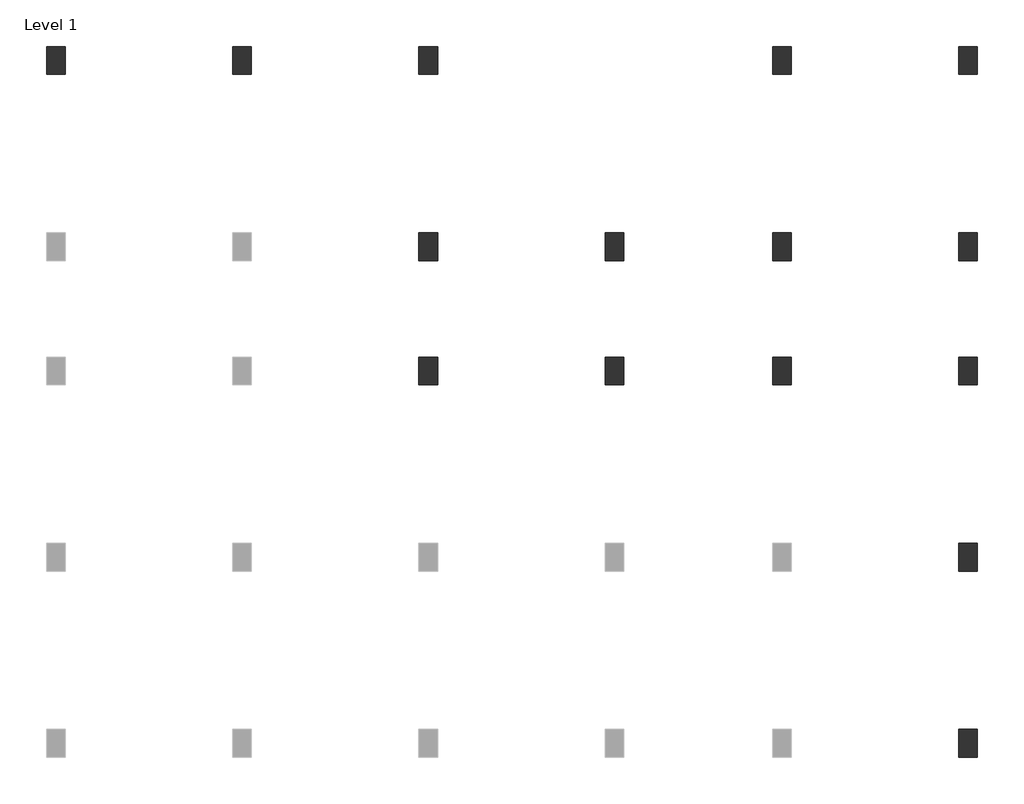
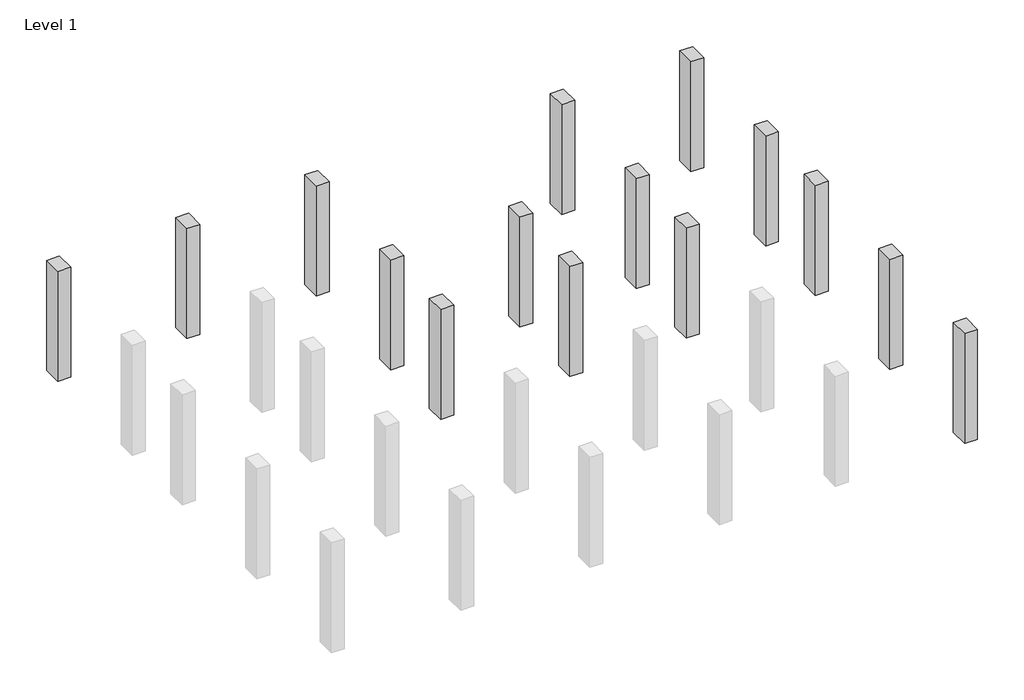
# One storey, part 2 of 2: 30 columns.
"""IFC4 building model written with IfcOpenShell, lengths in millimetres."""

from ifc_helpers import new_model, si_unit, frame, origin, place, context, project, spatial, polyline, outline, extrude, faceted_brep, element, save

model = new_model("IFC4")

# Units and contexts
model_context = context("Model", 3, world=origin())
ifc_project = project(units=[si_unit("LENGTHUNIT", "METRE", prefix="MILLI")], contexts=[model_context])

# Site, building, storey
site = spatial("IfcSite", under=ifc_project)
building = spatial("IfcBuilding", under=site)
storey = spatial("IfcBuildingStorey", under=building, Name="Level 1", Elevation=1219.2)

# Columns
placement = place(None, origin())
element("IfcColumn", 1, ObjectType="Concrete-Rectangular-Column : c1", at=placement, inside=storey, context=model_context, shape_type="SweptSolid", body=[
    extrude(outline(polyline([(2607.7603583, 7215.6647757), (2607.7603583, 7672.8647757), (2912.5603583, 7672.8647757), (2912.5603583, 7215.6647757), (2607.7603583, 7215.6647757)])), frame((0.0, 0.0, 1219.2), z_axis=(0.0, 0.0, 1.0), x_axis=(1.0, 0.0, 0.0)), (0.0, 0.0, 1.0), 2743.2),
])
element("IfcColumn", 2, ObjectType="Concrete-Rectangular-Column : c1", at=placement, inside=storey, context=model_context, shape_type="Brep", body=[
    faceted_brep([(2607.7603583, 10263.6647757, 1219.2), (2607.7603583, 10720.8647757, 1219.2), (2912.5603583, 10720.8647757, 1219.2), (2912.5603583, 10263.6647757, 1219.2), (2607.7603583, 10263.6647757, 3962.4), (2607.7603583, 10720.8647757, 3962.4), (2607.7603583, 10720.8647757, 2743.2), (2607.7603583, 10720.8647757, 2133.6), (2607.7603583, 10263.6647757, 2133.6), (2607.7603583, 10263.6647757, 2743.2), (2912.5603583, 10720.8647757, 3962.4), (2912.5603583, 10720.8647757, 2743.2), (2912.5603583, 10720.8647757, 2133.6), (2912.5603583, 10263.6647757, 3962.4), (2912.5603583, 10263.6647757, 2743.2), (2912.5603583, 10263.6647757, 2133.6)], [[[0, 1, 2, 3]], [[4, 5, 6, 7, 1, 0, 8, 9]], [[5, 10, 11, 12, 2, 1, 7, 6]], [[10, 13, 14, 15, 3, 2, 12, 11]], [[13, 4, 9, 8, 0, 3, 15, 14]], [[4, 13, 10, 5]]]),
])
element("IfcColumn", 3, ObjectType="Concrete-Rectangular-Column : c1", at=placement, inside=storey, context=model_context, shape_type="Brep", body=[
    faceted_brep([(-6231.4396417, 13311.6647757, 1219.2), (-6231.4396417, 13768.8647757, 1219.2), (-5926.6396417, 13768.8647757, 1219.2), (-5926.6396417, 13311.6647757, 1219.2), (-6231.4396417, 13311.6647757, 3962.4), (-6231.4396417, 13768.8647757, 3962.4), (-6231.4396417, 13768.8647757, 2743.2), (-6231.4396417, 13768.8647757, 2133.6), (-6231.4396417, 13311.6647757, 2133.6), (-6231.4396417, 13311.6647757, 2743.2), (-5926.6396417, 13768.8647757, 3962.4), (-5926.6396417, 13768.8647757, 2743.2), (-5926.6396417, 13768.8647757, 2133.6), (-5926.6396417, 13311.6647757, 3962.4), (-5926.6396417, 13311.6647757, 2743.2), (-5926.6396417, 13311.6647757, 2133.6)], [[[0, 1, 2, 3]], [[4, 5, 6, 7, 1, 0, 8, 9]], [[5, 10, 11, 12, 2, 1, 7, 6]], [[10, 13, 14, 15, 3, 2, 12, 11]], [[13, 4, 9, 8, 0, 3, 15, 14]], [[4, 13, 10, 5]]]),
])
element("IfcColumn", 4, ObjectType="Concrete-Rectangular-Column : c1", at=placement, inside=storey, context=model_context, shape_type="Brep", body=[
    faceted_brep([(-3183.4396417, 13311.6647757, 1219.2), (-3183.4396417, 13768.8647757, 1219.2), (-2878.6396417, 13768.8647757, 1219.2), (-2878.6396417, 13311.6647757, 1219.2), (-3183.4396417, 13311.6647757, 3962.4), (-3183.4396417, 13768.8647757, 3962.4), (-3183.4396417, 13768.8647757, 2743.2), (-3183.4396417, 13768.8647757, 2133.6), (-3183.4396417, 13311.6647757, 2133.6), (-3183.4396417, 13311.6647757, 2743.2), (-2878.6396417, 13768.8647757, 3962.4), (-2878.6396417, 13768.8647757, 2743.2), (-2878.6396417, 13768.8647757, 2133.6), (-2878.6396417, 13311.6647757, 3962.4), (-2878.6396417, 13311.6647757, 2743.2), (-2878.6396417, 13311.6647757, 2133.6)], [[[0, 1, 2, 3]], [[4, 5, 6, 7, 1, 0, 8, 9]], [[5, 10, 11, 12, 2, 1, 7, 6]], [[10, 13, 14, 15, 3, 2, 12, 11]], [[13, 4, 9, 8, 0, 3, 15, 14]], [[4, 13, 10, 5]]]),
])
element("IfcColumn", 5, ObjectType="Concrete-Rectangular-Column : c1", at=placement, inside=storey, context=model_context, shape_type="Brep", body=[
    faceted_brep([(-440.2396417, 13311.6647757, 1219.2), (-440.2396417, 13768.8647757, 1219.2), (-135.4396417, 13768.8647757, 1219.2), (-135.4396417, 13311.6647757, 1219.2), (-440.2396417, 13311.6647757, 3962.4), (-440.2396417, 13768.8647757, 3962.4), (-440.2396417, 13768.8647757, 2743.2), (-440.2396417, 13768.8647757, 2133.6), (-440.2396417, 13311.6647757, 2133.6), (-440.2396417, 13311.6647757, 2743.2), (-135.4396417, 13768.8647757, 3962.4), (-135.4396417, 13768.8647757, 2743.2), (-135.4396417, 13768.8647757, 2133.6), (-135.4396417, 13311.6647757, 3962.4), (-135.4396417, 13311.6647757, 2743.2), (-135.4396417, 13311.6647757, 2133.6)], [[[0, 1, 2, 3]], [[4, 5, 6, 7, 1, 0, 8, 9]], [[5, 10, 11, 12, 2, 1, 7, 6]], [[10, 13, 14, 15, 3, 2, 12, 11]], [[13, 4, 9, 8, 0, 3, 15, 14]], [[4, 13, 10, 5]]]),
])
element("IfcColumn", 6, ObjectType="Concrete-Rectangular-Column : c1", at=placement, inside=storey, context=model_context, shape_type="Brep", body=[
    faceted_brep([(2607.7603583, 13311.6647757, 1219.2), (2607.7603583, 13768.8647757, 1219.2), (2912.5603583, 13768.8647757, 1219.2), (2912.5603583, 13311.6647757, 1219.2), (2607.7603583, 13311.6647757, 3962.4), (2607.7603583, 13768.8647757, 3962.4), (2607.7603583, 13768.8647757, 2743.2), (2607.7603583, 13768.8647757, 2133.6), (2607.7603583, 13311.6647757, 2133.6), (2607.7603583, 13311.6647757, 2743.2), (2912.5603583, 13768.8647757, 3962.4), (2912.5603583, 13768.8647757, 2743.2), (2912.5603583, 13768.8647757, 2133.6), (2912.5603583, 13311.6647757, 3962.4), (2912.5603583, 13311.6647757, 2743.2), (2912.5603583, 13311.6647757, 2133.6)], [[[0, 1, 2, 3]], [[4, 5, 6, 7, 1, 0, 8, 9]], [[5, 10, 11, 12, 2, 1, 7, 6]], [[10, 13, 14, 15, 3, 2, 12, 11]], [[13, 4, 9, 8, 0, 3, 15, 14]], [[4, 13, 10, 5]]]),
])
element("IfcColumn", 7, ObjectType="Concrete-Rectangular-Column : c1", at=placement, inside=storey, context=model_context, shape_type="Brep", body=[
    faceted_brep([(-6231.4396417, 15346.9119241, 1219.2), (-6231.4396417, 15804.1119241, 1219.2), (-5926.6396417, 15804.1119241, 1219.2), (-5926.6396417, 15346.9119241, 1219.2), (-6231.4396417, 15346.9119241, 3962.4), (-6231.4396417, 15804.1119241, 3962.4), (-6231.4396417, 15804.1119241, 2743.2), (-6231.4396417, 15804.1119241, 2133.6), (-6231.4396417, 15346.9119241, 2133.6), (-6231.4396417, 15346.9119241, 2743.2), (-5926.6396417, 15804.1119241, 3962.4), (-5926.6396417, 15804.1119241, 2743.2), (-5926.6396417, 15804.1119241, 2133.6), (-5926.6396417, 15346.9119241, 3962.4), (-5926.6396417, 15346.9119241, 2743.2), (-5926.6396417, 15346.9119241, 2133.6)], [[[0, 1, 2, 3]], [[4, 5, 6, 7, 1, 0, 8, 9]], [[5, 10, 11, 12, 2, 1, 7, 6]], [[10, 13, 14, 15, 3, 2, 12, 11]], [[13, 4, 9, 8, 0, 3, 15, 14]], [[4, 13, 10, 5]]]),
])
element("IfcColumn", 8, ObjectType="Concrete-Rectangular-Column : c1", at=placement, inside=storey, context=model_context, shape_type="Brep", body=[
    faceted_brep([(-3183.4396417, 15346.9119241, 1219.2), (-3183.4396417, 15804.1119241, 1219.2), (-2878.6396417, 15804.1119241, 1219.2), (-2878.6396417, 15346.9119241, 1219.2), (-3183.4396417, 15346.9119241, 3962.4), (-3183.4396417, 15804.1119241, 3962.4), (-3183.4396417, 15804.1119241, 2743.2), (-3183.4396417, 15804.1119241, 2133.6), (-3183.4396417, 15346.9119241, 2133.6), (-3183.4396417, 15346.9119241, 2743.2), (-2878.6396417, 15804.1119241, 3962.4), (-2878.6396417, 15804.1119241, 2743.2), (-2878.6396417, 15804.1119241, 2133.6), (-2878.6396417, 15346.9119241, 3962.4), (-2878.6396417, 15346.9119241, 2743.2), (-2878.6396417, 15346.9119241, 2133.6)], [[[0, 1, 2, 3]], [[4, 5, 6, 7, 1, 0, 8, 9]], [[5, 10, 11, 12, 2, 1, 7, 6]], [[10, 13, 14, 15, 3, 2, 12, 11]], [[13, 4, 9, 8, 0, 3, 15, 14]], [[4, 13, 10, 5]]]),
])
element("IfcColumn", 9, ObjectType="Concrete-Rectangular-Column : c1", at=placement, inside=storey, context=model_context, shape_type="Brep", body=[
    faceted_brep([(-440.2396417, 15346.9119241, 1219.2), (-440.2396417, 15804.1119241, 1219.2), (-135.4396417, 15804.1119241, 1219.2), (-135.4396417, 15346.9119241, 1219.2), (-440.2396417, 15346.9119241, 3962.4), (-440.2396417, 15804.1119241, 3962.4), (-440.2396417, 15804.1119241, 2743.2), (-440.2396417, 15804.1119241, 2133.6), (-440.2396417, 15346.9119241, 2133.6), (-440.2396417, 15346.9119241, 2743.2), (-135.4396417, 15804.1119241, 3962.4), (-135.4396417, 15804.1119241, 2743.2), (-135.4396417, 15804.1119241, 2133.6), (-135.4396417, 15346.9119241, 3962.4), (-135.4396417, 15346.9119241, 2743.2), (-135.4396417, 15346.9119241, 2133.6)], [[[0, 1, 2, 3]], [[4, 5, 6, 7, 1, 0, 8, 9]], [[5, 10, 11, 12, 2, 1, 7, 6]], [[10, 13, 14, 15, 3, 2, 12, 11]], [[13, 4, 9, 8, 0, 3, 15, 14]], [[4, 13, 10, 5]]]),
])
element("IfcColumn", 10, ObjectType="Concrete-Rectangular-Column : c1", at=placement, inside=storey, context=model_context, shape_type="Brep", body=[
    faceted_brep([(2607.7603583, 15346.9119241, 1219.2), (2607.7603583, 15804.1119241, 1219.2), (2912.5603583, 15804.1119241, 1219.2), (2912.5603583, 15346.9119241, 1219.2), (2607.7603583, 15346.9119241, 3962.4), (2607.7603583, 15804.1119241, 3962.4), (2607.7603583, 15804.1119241, 2743.2), (2607.7603583, 15804.1119241, 2133.6), (2607.7603583, 15346.9119241, 2133.6), (2607.7603583, 15346.9119241, 2743.2), (2912.5603583, 15804.1119241, 3962.4), (2912.5603583, 15804.1119241, 2743.2), (2912.5603583, 15804.1119241, 2133.6), (2912.5603583, 15346.9119241, 3962.4), (2912.5603583, 15346.9119241, 2743.2), (2912.5603583, 15346.9119241, 2133.6)], [[[0, 1, 2, 3]], [[4, 5, 6, 7, 1, 0, 8, 9]], [[5, 10, 11, 12, 2, 1, 7, 6]], [[10, 13, 14, 15, 3, 2, 12, 11]], [[13, 4, 9, 8, 0, 3, 15, 14]], [[4, 13, 10, 5]]]),
])
element("IfcColumn", 11, ObjectType="Concrete-Rectangular-Column : c1", at=placement, inside=storey, context=model_context, shape_type="SweptSolid", body=[
    extrude(outline(polyline([(-12327.4396417, 18394.9119241), (-12327.4396417, 18852.1119241), (-12022.6396417, 18852.1119241), (-12022.6396417, 18394.9119241), (-12327.4396417, 18394.9119241)])), frame((0.0, 0.0, 1219.2), z_axis=(0.0, 0.0, 1.0), x_axis=(1.0, 0.0, 0.0)), (0.0, 0.0, 1.0), 2743.2),
])
element("IfcColumn", 12, ObjectType="Concrete-Rectangular-Column : c1", at=placement, inside=storey, context=model_context, shape_type="SweptSolid", body=[
    extrude(outline(polyline([(-9279.4396417, 18394.9119241), (-9279.4396417, 18852.1119241), (-8974.6396417, 18852.1119241), (-8974.6396417, 18394.9119241), (-9279.4396417, 18394.9119241)])), frame((0.0, 0.0, 1219.2), z_axis=(0.0, 0.0, 1.0), x_axis=(1.0, 0.0, 0.0)), (0.0, 0.0, 1.0), 2743.2),
])
element("IfcColumn", 13, ObjectType="Concrete-Rectangular-Column : c1", at=placement, inside=storey, context=model_context, shape_type="SweptSolid", body=[
    extrude(outline(polyline([(-6231.4396417, 18394.9119241), (-6231.4396417, 18852.1119241), (-5926.6396417, 18852.1119241), (-5926.6396417, 18394.9119241), (-6231.4396417, 18394.9119241)])), frame((0.0, 0.0, 1219.2), z_axis=(0.0, 0.0, 1.0), x_axis=(1.0, 0.0, 0.0)), (0.0, 0.0, 1.0), 2743.2),
])
element("IfcColumn", 14, ObjectType="Concrete-Rectangular-Column : c1", at=placement, inside=storey, context=model_context, shape_type="SweptSolid", body=[
    extrude(outline(polyline([(-440.2396417, 18394.9119241), (-440.2396417, 18852.1119241), (-135.4396417, 18852.1119241), (-135.4396417, 18394.9119241), (-440.2396417, 18394.9119241)])), frame((0.0, 0.0, 1219.2), z_axis=(0.0, 0.0, 1.0), x_axis=(1.0, 0.0, 0.0)), (0.0, 0.0, 1.0), 2743.2),
])
element("IfcColumn", 15, ObjectType="Concrete-Rectangular-Column : c1", at=placement, inside=storey, context=model_context, shape_type="SweptSolid", body=[
    extrude(outline(polyline([(2607.7603583, 18394.9119241), (2607.7603583, 18852.1119241), (2912.5603583, 18852.1119241), (2912.5603583, 18394.9119241), (2607.7603583, 18394.9119241)])), frame((0.0, 0.0, 1219.2), z_axis=(0.0, 0.0, 1.0), x_axis=(1.0, 0.0, 0.0)), (0.0, 0.0, 1.0), 2743.2),
])
element("IfcColumn", 16, ObjectType="Concrete-Rectangular-Column : c1", at=placement, inside=storey, context=model_context, shape_type="Brep", body=[
    faceted_brep([(2607.7603583, 7215.6647757, 1219.2), (2607.7603583, 7672.8647757, 1219.2), (2912.5603583, 7672.8647757, 1219.2), (2912.5603583, 7215.6647757, 1219.2), (2607.7603583, 7215.6647757, 3962.4), (2607.7603583, 7672.8647757, 3962.4), (2607.7603583, 7672.8647757, 2743.2), (2607.7603583, 7672.8647757, 2133.6), (2912.5603583, 7672.8647757, 3962.4), (2912.5603583, 7672.8647757, 2743.2), (2912.5603583, 7672.8647757, 2133.6), (2912.5603583, 7215.6647757, 3962.4)], [[[0, 1, 2, 3]], [[4, 5, 6, 7, 1, 0]], [[5, 8, 9, 10, 2, 1, 7, 6]], [[8, 11, 3, 2, 10, 9]], [[11, 4, 0, 3]], [[4, 11, 8, 5]]]),
])
element("IfcColumn", 17, ObjectType="Concrete-Rectangular-Column : c1", at=placement, inside=storey, context=model_context, shape_type="Brep", body=[
    faceted_brep([(2607.7603583, 10263.6647757, 1219.2), (2607.7603583, 10720.8647757, 1219.2), (2912.5603583, 10720.8647757, 1219.2), (2912.5603583, 10263.6647757, 1219.2), (2607.7603583, 10263.6647757, 3962.4), (2607.7603583, 10720.8647757, 3962.4), (2607.7603583, 10720.8647757, 2743.2), (2607.7603583, 10720.8647757, 2133.6), (2607.7603583, 10263.6647757, 2133.6), (2607.7603583, 10263.6647757, 2743.2), (2912.5603583, 10720.8647757, 3962.4), (2912.5603583, 10720.8647757, 2743.2), (2912.5603583, 10720.8647757, 2133.6), (2912.5603583, 10263.6647757, 3962.4), (2912.5603583, 10263.6647757, 2743.2), (2912.5603583, 10263.6647757, 2133.6)], [[[0, 1, 2, 3]], [[4, 5, 6, 7, 1, 0, 8, 9]], [[5, 10, 11, 12, 2, 1, 7, 6]], [[10, 13, 14, 15, 3, 2, 12, 11]], [[13, 4, 9, 8, 0, 3, 15, 14]], [[4, 13, 10, 5]]]),
])
element("IfcColumn", 18, ObjectType="Concrete-Rectangular-Column : c1", at=placement, inside=storey, context=model_context, shape_type="Brep", body=[
    faceted_brep([(-6231.4396417, 13311.6647757, 1219.2), (-6231.4396417, 13768.8647757, 1219.2), (-5926.6396417, 13768.8647757, 1219.2), (-5926.6396417, 13311.6647757, 1219.2), (-6231.4396417, 13311.6647757, 3962.4), (-6231.4396417, 13768.8647757, 3962.4), (-6231.4396417, 13768.8647757, 2743.2), (-6231.4396417, 13768.8647757, 2133.6), (-6231.4396417, 13311.6647757, 2133.6), (-6231.4396417, 13311.6647757, 2743.2), (-5926.6396417, 13768.8647757, 3962.4), (-5926.6396417, 13768.8647757, 2743.2), (-5926.6396417, 13768.8647757, 2133.6), (-5926.6396417, 13311.6647757, 3962.4), (-5926.6396417, 13311.6647757, 2743.2), (-5926.6396417, 13311.6647757, 2133.6)], [[[0, 1, 2, 3]], [[4, 5, 6, 7, 1, 0, 8, 9]], [[5, 10, 11, 12, 2, 1, 7, 6]], [[10, 13, 14, 15, 3, 2, 12, 11]], [[13, 4, 9, 8, 0, 3, 15, 14]], [[4, 13, 10, 5]]]),
])
element("IfcColumn", 19, ObjectType="Concrete-Rectangular-Column : c1", at=placement, inside=storey, context=model_context, shape_type="Brep", body=[
    faceted_brep([(-3183.4396417, 13311.6647757, 1219.2), (-3183.4396417, 13768.8647757, 1219.2), (-2878.6396417, 13768.8647757, 1219.2), (-2878.6396417, 13311.6647757, 1219.2), (-3183.4396417, 13311.6647757, 3962.4), (-3183.4396417, 13768.8647757, 3962.4), (-3183.4396417, 13768.8647757, 2743.2), (-3183.4396417, 13768.8647757, 2133.6), (-3183.4396417, 13311.6647757, 2133.6), (-3183.4396417, 13311.6647757, 2743.2), (-2878.6396417, 13768.8647757, 3962.4), (-2878.6396417, 13768.8647757, 2743.2), (-2878.6396417, 13768.8647757, 2133.6), (-2878.6396417, 13311.6647757, 3962.4), (-2878.6396417, 13311.6647757, 2743.2), (-2878.6396417, 13311.6647757, 2133.6)], [[[0, 1, 2, 3]], [[4, 5, 6, 7, 1, 0, 8, 9]], [[5, 10, 11, 12, 2, 1, 7, 6]], [[10, 13, 14, 15, 3, 2, 12, 11]], [[13, 4, 9, 8, 0, 3, 15, 14]], [[4, 13, 10, 5]]]),
])
element("IfcColumn", 20, ObjectType="Concrete-Rectangular-Column : c1", at=placement, inside=storey, context=model_context, shape_type="Brep", body=[
    faceted_brep([(-440.2396417, 13311.6647757, 1219.2), (-440.2396417, 13768.8647757, 1219.2), (-135.4396417, 13768.8647757, 1219.2), (-135.4396417, 13311.6647757, 1219.2), (-440.2396417, 13311.6647757, 3962.4), (-440.2396417, 13768.8647757, 3962.4), (-440.2396417, 13768.8647757, 2743.2), (-440.2396417, 13768.8647757, 2133.6), (-440.2396417, 13311.6647757, 2133.6), (-440.2396417, 13311.6647757, 2743.2), (-135.4396417, 13768.8647757, 3962.4), (-135.4396417, 13768.8647757, 2743.2), (-135.4396417, 13768.8647757, 2133.6), (-135.4396417, 13311.6647757, 3962.4), (-135.4396417, 13311.6647757, 2743.2), (-135.4396417, 13311.6647757, 2133.6)], [[[0, 1, 2, 3]], [[4, 5, 6, 7, 1, 0, 8, 9]], [[5, 10, 11, 12, 2, 1, 7, 6]], [[10, 13, 14, 15, 3, 2, 12, 11]], [[13, 4, 9, 8, 0, 3, 15, 14]], [[4, 13, 10, 5]]]),
])
element("IfcColumn", 21, ObjectType="Concrete-Rectangular-Column : c1", at=placement, inside=storey, context=model_context, shape_type="Brep", body=[
    faceted_brep([(2607.7603583, 13311.6647757, 1219.2), (2607.7603583, 13768.8647757, 1219.2), (2912.5603583, 13768.8647757, 1219.2), (2912.5603583, 13311.6647757, 1219.2), (2607.7603583, 13311.6647757, 3962.4), (2607.7603583, 13768.8647757, 3962.4), (2607.7603583, 13768.8647757, 2743.2), (2607.7603583, 13768.8647757, 2133.6), (2607.7603583, 13311.6647757, 2133.6), (2607.7603583, 13311.6647757, 2743.2), (2912.5603583, 13768.8647757, 3962.4), (2912.5603583, 13768.8647757, 2743.2), (2912.5603583, 13768.8647757, 2133.6), (2912.5603583, 13311.6647757, 3962.4), (2912.5603583, 13311.6647757, 2743.2), (2912.5603583, 13311.6647757, 2133.6)], [[[0, 1, 2, 3]], [[4, 5, 6, 7, 1, 0, 8, 9]], [[5, 10, 11, 12, 2, 1, 7, 6]], [[10, 13, 14, 15, 3, 2, 12, 11]], [[13, 4, 9, 8, 0, 3, 15, 14]], [[4, 13, 10, 5]]]),
])
element("IfcColumn", 22, ObjectType="Concrete-Rectangular-Column : c1", at=placement, inside=storey, context=model_context, shape_type="Brep", body=[
    faceted_brep([(-6231.4396417, 15346.9119241, 1219.2), (-6231.4396417, 15804.1119241, 1219.2), (-5926.6396417, 15804.1119241, 1219.2), (-5926.6396417, 15346.9119241, 1219.2), (-6231.4396417, 15346.9119241, 3962.4), (-6231.4396417, 15804.1119241, 3962.4), (-6231.4396417, 15804.1119241, 2743.2), (-6231.4396417, 15804.1119241, 2133.6), (-6231.4396417, 15346.9119241, 2133.6), (-6231.4396417, 15346.9119241, 2743.2), (-5926.6396417, 15804.1119241, 3962.4), (-5926.6396417, 15804.1119241, 2743.2), (-5926.6396417, 15804.1119241, 2133.6), (-5926.6396417, 15346.9119241, 3962.4), (-5926.6396417, 15346.9119241, 2743.2), (-5926.6396417, 15346.9119241, 2133.6)], [[[0, 1, 2, 3]], [[4, 5, 6, 7, 1, 0, 8, 9]], [[5, 10, 11, 12, 2, 1, 7, 6]], [[10, 13, 14, 15, 3, 2, 12, 11]], [[13, 4, 9, 8, 0, 3, 15, 14]], [[4, 13, 10, 5]]]),
])
element("IfcColumn", 23, ObjectType="Concrete-Rectangular-Column : c1", at=placement, inside=storey, context=model_context, shape_type="Brep", body=[
    faceted_brep([(-3183.4396417, 15346.9119241, 1219.2), (-3183.4396417, 15804.1119241, 1219.2), (-2878.6396417, 15804.1119241, 1219.2), (-2878.6396417, 15346.9119241, 1219.2), (-3183.4396417, 15346.9119241, 3962.4), (-3183.4396417, 15804.1119241, 3962.4), (-3183.4396417, 15804.1119241, 2743.2), (-3183.4396417, 15804.1119241, 2133.6), (-3183.4396417, 15346.9119241, 2133.6), (-3183.4396417, 15346.9119241, 2743.2), (-2878.6396417, 15804.1119241, 3962.4), (-2878.6396417, 15804.1119241, 2743.2), (-2878.6396417, 15804.1119241, 2133.6), (-2878.6396417, 15346.9119241, 3962.4), (-2878.6396417, 15346.9119241, 2743.2), (-2878.6396417, 15346.9119241, 2133.6)], [[[0, 1, 2, 3]], [[4, 5, 6, 7, 1, 0, 8, 9]], [[5, 10, 11, 12, 2, 1, 7, 6]], [[10, 13, 14, 15, 3, 2, 12, 11]], [[13, 4, 9, 8, 0, 3, 15, 14]], [[4, 13, 10, 5]]]),
])
element("IfcColumn", 24, ObjectType="Concrete-Rectangular-Column : c1", at=placement, inside=storey, context=model_context, shape_type="Brep", body=[
    faceted_brep([(-440.2396417, 15346.9119241, 1219.2), (-440.2396417, 15804.1119241, 1219.2), (-135.4396417, 15804.1119241, 1219.2), (-135.4396417, 15346.9119241, 1219.2), (-440.2396417, 15346.9119241, 3962.4), (-440.2396417, 15804.1119241, 3962.4), (-440.2396417, 15804.1119241, 2743.2), (-440.2396417, 15804.1119241, 2133.6), (-440.2396417, 15346.9119241, 2133.6), (-440.2396417, 15346.9119241, 2743.2), (-135.4396417, 15804.1119241, 3962.4), (-135.4396417, 15804.1119241, 2743.2), (-135.4396417, 15804.1119241, 2133.6), (-135.4396417, 15346.9119241, 3962.4), (-135.4396417, 15346.9119241, 2743.2), (-135.4396417, 15346.9119241, 2133.6)], [[[0, 1, 2, 3]], [[4, 5, 6, 7, 1, 0, 8, 9]], [[5, 10, 11, 12, 2, 1, 7, 6]], [[10, 13, 14, 15, 3, 2, 12, 11]], [[13, 4, 9, 8, 0, 3, 15, 14]], [[4, 13, 10, 5]]]),
])
element("IfcColumn", 25, ObjectType="Concrete-Rectangular-Column : c1", at=placement, inside=storey, context=model_context, shape_type="Brep", body=[
    faceted_brep([(2607.7603583, 15346.9119241, 1219.2), (2607.7603583, 15804.1119241, 1219.2), (2912.5603583, 15804.1119241, 1219.2), (2912.5603583, 15346.9119241, 1219.2), (2607.7603583, 15346.9119241, 3962.4), (2607.7603583, 15804.1119241, 3962.4), (2607.7603583, 15804.1119241, 2743.2), (2607.7603583, 15804.1119241, 2133.6), (2607.7603583, 15346.9119241, 2133.6), (2607.7603583, 15346.9119241, 2743.2), (2912.5603583, 15804.1119241, 3962.4), (2912.5603583, 15804.1119241, 2743.2), (2912.5603583, 15804.1119241, 2133.6), (2912.5603583, 15346.9119241, 3962.4), (2912.5603583, 15346.9119241, 2743.2), (2912.5603583, 15346.9119241, 2133.6)], [[[0, 1, 2, 3]], [[4, 5, 6, 7, 1, 0, 8, 9]], [[5, 10, 11, 12, 2, 1, 7, 6]], [[10, 13, 14, 15, 3, 2, 12, 11]], [[13, 4, 9, 8, 0, 3, 15, 14]], [[4, 13, 10, 5]]]),
])
element("IfcColumn", 26, ObjectType="Concrete-Rectangular-Column : c1", at=placement, inside=storey, context=model_context, shape_type="Brep", body=[
    faceted_brep([(-12327.4396417, 18394.9119241, 1219.2), (-12327.4396417, 18852.1119241, 1219.2), (-12022.6396417, 18852.1119241, 1219.2), (-12022.6396417, 18394.9119241, 1219.2), (-12327.4396417, 18394.9119241, 3962.4), (-12327.4396417, 18852.1119241, 3962.4), (-12327.4396417, 18394.9119241, 2133.6), (-12327.4396417, 18394.9119241, 2743.2), (-12022.6396417, 18852.1119241, 3962.4), (-12022.6396417, 18394.9119241, 3962.4), (-12022.6396417, 18394.9119241, 2743.2), (-12022.6396417, 18394.9119241, 2133.6)], [[[0, 1, 2, 3]], [[4, 5, 1, 0, 6, 7]], [[5, 8, 2, 1]], [[8, 9, 10, 11, 3, 2]], [[9, 4, 7, 6, 0, 3, 11, 10]], [[4, 9, 8, 5]]]),
])
element("IfcColumn", 27, ObjectType="Concrete-Rectangular-Column : c1", at=placement, inside=storey, context=model_context, shape_type="Brep", body=[
    faceted_brep([(-9279.4396417, 18394.9119241, 1219.2), (-9279.4396417, 18852.1119241, 1219.2), (-8974.6396417, 18852.1119241, 1219.2), (-8974.6396417, 18394.9119241, 1219.2), (-9279.4396417, 18394.9119241, 3962.4), (-9279.4396417, 18852.1119241, 3962.4), (-9279.4396417, 18394.9119241, 2133.6), (-9279.4396417, 18394.9119241, 2743.2), (-8974.6396417, 18852.1119241, 3962.4), (-8974.6396417, 18394.9119241, 3962.4), (-8974.6396417, 18394.9119241, 2743.2), (-8974.6396417, 18394.9119241, 2133.6)], [[[0, 1, 2, 3]], [[4, 5, 1, 0, 6, 7]], [[5, 8, 2, 1]], [[8, 9, 10, 11, 3, 2]], [[9, 4, 7, 6, 0, 3, 11, 10]], [[4, 9, 8, 5]]]),
])
element("IfcColumn", 28, ObjectType="Concrete-Rectangular-Column : c1", at=placement, inside=storey, context=model_context, shape_type="Brep", body=[
    faceted_brep([(-6231.4396417, 18394.9119241, 1219.2), (-6231.4396417, 18852.1119241, 1219.2), (-5926.6396417, 18852.1119241, 1219.2), (-5926.6396417, 18394.9119241, 1219.2), (-6231.4396417, 18394.9119241, 3962.4), (-6231.4396417, 18852.1119241, 3962.4), (-6231.4396417, 18394.9119241, 2133.6), (-6231.4396417, 18394.9119241, 2743.2), (-5926.6396417, 18852.1119241, 3962.4), (-5926.6396417, 18394.9119241, 3962.4), (-5926.6396417, 18394.9119241, 2743.2), (-5926.6396417, 18394.9119241, 2133.6)], [[[0, 1, 2, 3]], [[4, 5, 1, 0, 6, 7]], [[5, 8, 2, 1]], [[8, 9, 10, 11, 3, 2]], [[9, 4, 7, 6, 0, 3, 11, 10]], [[4, 9, 8, 5]]]),
])
element("IfcColumn", 29, ObjectType="Concrete-Rectangular-Column : c1", at=placement, inside=storey, context=model_context, shape_type="Brep", body=[
    faceted_brep([(-440.2396417, 18394.9119241, 1219.2), (-440.2396417, 18852.1119241, 1219.2), (-135.4396417, 18852.1119241, 1219.2), (-135.4396417, 18394.9119241, 1219.2), (-440.2396417, 18394.9119241, 3962.4), (-440.2396417, 18852.1119241, 3962.4), (-440.2396417, 18394.9119241, 2133.6), (-440.2396417, 18394.9119241, 2743.2), (-135.4396417, 18852.1119241, 3962.4), (-135.4396417, 18394.9119241, 3962.4), (-135.4396417, 18394.9119241, 2743.2), (-135.4396417, 18394.9119241, 2133.6)], [[[0, 1, 2, 3]], [[4, 5, 1, 0, 6, 7]], [[5, 8, 2, 1]], [[8, 9, 10, 11, 3, 2]], [[9, 4, 7, 6, 0, 3, 11, 10]], [[4, 9, 8, 5]]]),
])
element("IfcColumn", 30, ObjectType="Concrete-Rectangular-Column : c1", at=placement, inside=storey, context=model_context, shape_type="Brep", body=[
    faceted_brep([(2607.7603583, 18394.9119241, 1219.2), (2607.7603583, 18852.1119241, 1219.2), (2912.5603583, 18852.1119241, 1219.2), (2912.5603583, 18394.9119241, 1219.2), (2607.7603583, 18394.9119241, 3962.4), (2607.7603583, 18852.1119241, 3962.4), (2607.7603583, 18394.9119241, 2133.6), (2607.7603583, 18394.9119241, 2743.2), (2912.5603583, 18852.1119241, 3962.4), (2912.5603583, 18394.9119241, 3962.4), (2912.5603583, 18394.9119241, 2743.2), (2912.5603583, 18394.9119241, 2133.6)], [[[0, 1, 2, 3]], [[4, 5, 1, 0, 6, 7]], [[5, 8, 2, 1]], [[8, 9, 10, 11, 3, 2]], [[9, 4, 7, 6, 0, 3, 11, 10]], [[4, 9, 8, 5]]]),
])

save(model, "model.ifc")

# Revit data of these elements
# Type "Concrete-Rectangular-Column : c1"
#   Assembly Code = "B10"
#   b = 1' - 0"
#   h = 1' - 6"
#   Structural Material [instance default] = Concrete, Cast-in-Place gray
# Elements 1, 2, 3, 4, 5, 6, 7, 8, 9, 10, 11, 12, 13, 14, 15, 16, 17, 18, 19, 20, 21, 22, 23, 24, 25, 26, 27, 28, 29, 30 (IfcColumn, "Concrete-Rectangular-Column : c1")
#   Comments = ""
#   Structural Material = Concrete, Cast-in-Place gray
#   Phase Created = New Construction
#   Materials on its faces: "Concrete, Cast-in-Place gray"
# Materials
#   "Concrete, Cast-in-Place gray": class "Concrete", colour RGB 192 192 192, transparency 0, Description = "Cast-in-place concrete", Cost = 0
